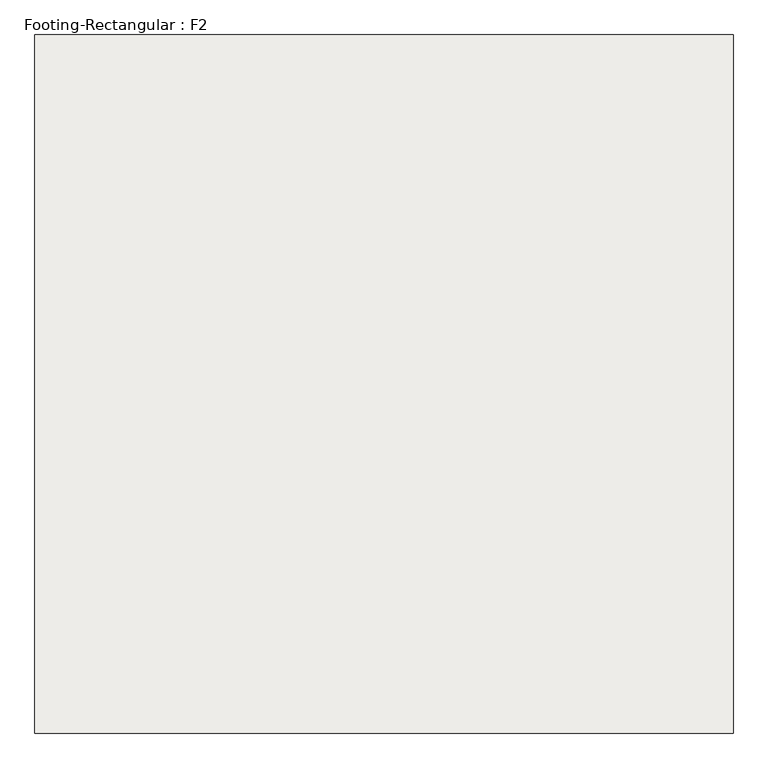
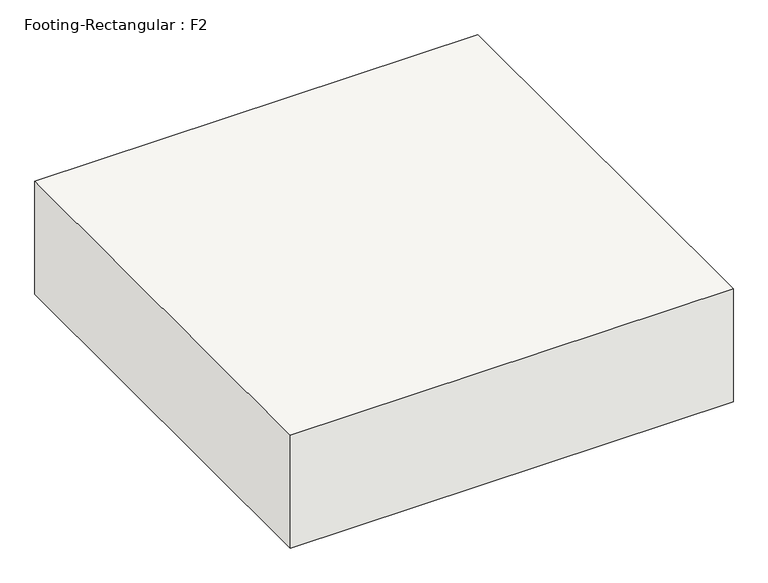
"""IFC4 building model written with IfcOpenShell, lengths in millimetres: slab geometry, Footing-Rectangular : F2."""

from ifc_helpers import new_model, si_unit, frame, origin, place, context, project, spatial, polyline, outline, extrude, source, transform, mapped, element, save


def footing_rectangular_f2_e38db0b8(model_context):
    return source(origin(), model_context, "Body", "SweptSolid", [
        extrude(outline(polyline([(990.6, 990.6), (990.6, -990.6), (-990.6, -990.6), (-990.6, 990.6), (990.6, 990.6)])), frame((0.0, 0.0, -533.4), z_axis=(0.0, 0.0, 1.0), x_axis=(1.0, 0.0, 0.0)), (0.0, 0.0, 1.0), 533.4),
    ])


if __name__ == "__main__":
    model = new_model("IFC4")
    model_context = context("Model", 3, world=origin())
    ifc_project = project(units=[si_unit("LENGTHUNIT", "METRE", prefix="MILLI")], contexts=[model_context])
    site = spatial("IfcSite", under=ifc_project)
    building = spatial("IfcBuilding", under=site)
    placement = place(None, origin())
    footing_rectangular_f2_shape = footing_rectangular_f2_e38db0b8(model_context)
    element("IfcSlab", 1, ObjectType="Footing-Rectangular : F2", at=placement, inside=building, context=model_context, shape_type="MappedRepresentation", body=[
        mapped(footing_rectangular_f2_shape, transform((0.0, 0.0, 0.0), x_axis=(1.0, 0.0, 0.0), y_axis=(0.0, 1.0, 0.0), z_axis=(0.0, 0.0, 1.0))),
    ])
    save(model, "model.ifc")

# Revit data of these elements
# Type "Footing-Rectangular : F2"
#   Width = 1981.2 mm
#   Length = 1981.2 mm
#   Foundation Thickness = 533.4 mm
#   Structural Material [instance default] = Concrete - Cast-in-Place Concrete
#   Assembly Code = ""
# Element 1 (IfcSlab, "Footing-Rectangular : F2")
#   Materials on its faces: "Concrete - Cast-in-Place Concrete"
# Materials
#   "Concrete - Cast-in-Place Concrete": class "Concrete", colour RGB 192 192 192, transparency 0, Cost = 0
